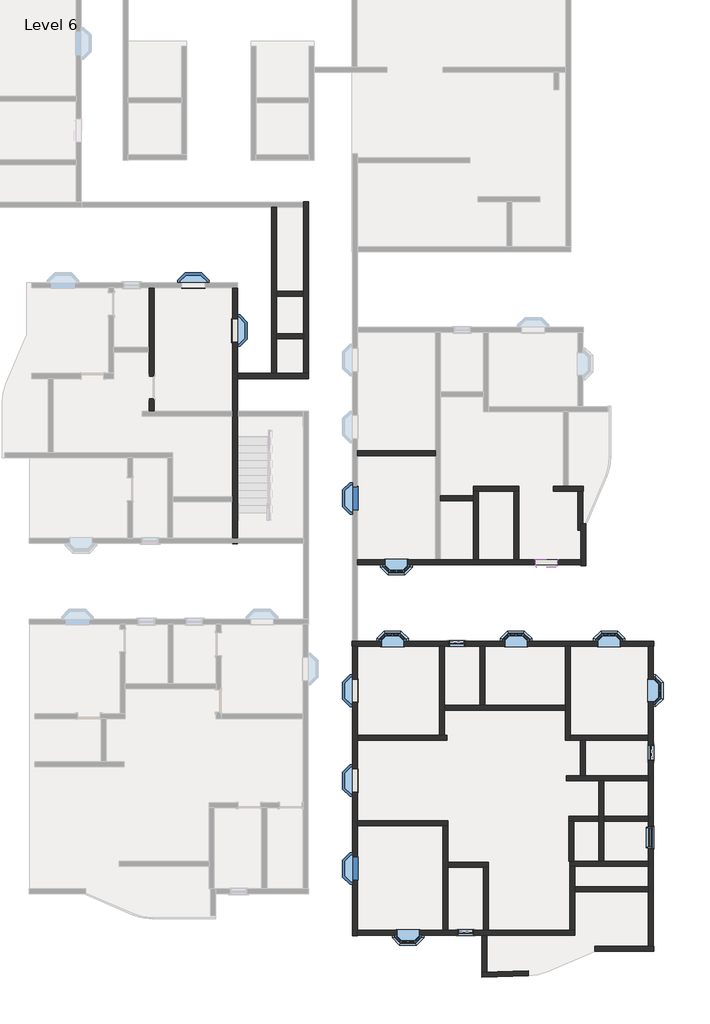
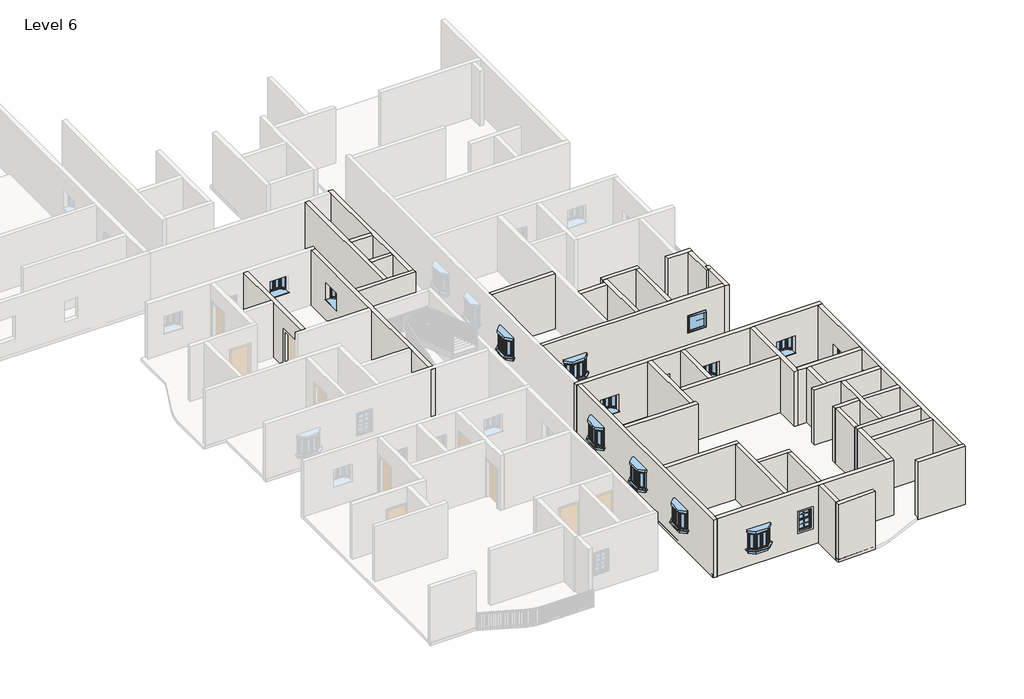
# One storey, part 2 of 14: 41 walls, 17 windows.
# Revit data of these elements (continued)
# Element 41 (IfcWall, "9\" w") (continued)
#   Phase Created = New Construction
#   Base Constraint = Level 6
#   Top Constraint = Level 7
#   Materials on its faces: "Default Wall", "Acoustic Ceiling Tile 24 x 24"
# Element 42 (IfcWindow, "910x910mm")
#   Mark = "314"
#   Phase Created = New Construction
#   Materials on its faces: "Window Frame", "Glass"
# Element 43 (IfcWindow, "910x910mm")
#   Mark = "316"
#   Phase Created = New Construction
#   Materials on its faces: "Window Frame", "Glass"
# Element 44 (IfcWindow, "910x910mm")
#   Mark = "334"
#   Phase Created = New Construction
#   Materials on its faces: "Window Frame", "Glass"
# Element 45 (IfcWindow, "910x910mm")
#   Mark = "325"
#   Phase Created = New Construction
#   Materials on its faces: "Window Frame", "Glass"
# Element 46 (IfcWindow, "910x910mm")
#   Mark = "326"
#   Phase Created = New Construction
#   Materials on its faces: "Window Frame", "Glass"
# Element 47 (IfcWindow, "910x910mm")
#   Mark = "327"
#   Phase Created = New Construction
#   Materials on its faces: "Window Frame", "Glass"
# Element 48 (IfcWindow, "910x910mm")
#   Mark = "328"
#   Phase Created = New Construction
#   Materials on its faces: "Window Frame", "Glass"
# Element 49 (IfcWindow, "910x910mm")
#   Mark = "329"
#   Phase Created = New Construction
#   Materials on its faces: "Window Frame", "Glass"
# Element 50 (IfcWindow, "910x910mm")
#   Mark = "330"
#   Phase Created = New Construction
#   Materials on its faces: "Window Frame", "Glass"
# Element 51 (IfcWindow, "910x910mm")
#   Mark = "331"
#   Phase Created = New Construction
#   Materials on its faces: "Window Frame", "Glass"
# Element 52 (IfcWindow, "910x910mm")
#   Mark = "332"
#   Phase Created = New Construction
#   Materials on its faces: "Window Frame", "Glass"
# Element 53 (IfcWindow, "910x910mm")
#   Mark = "333"
#   Phase Created = New Construction
#   Materials on its faces: "Window Frame", "Glass"
# Element 54 (IfcWindow, "Window-Double-Hung : 26\" x 42\"")
#   Mark = "356"
#   Window Inset = 0' - 0"
#   Interior Wall Closure = 0' - 1 1/2"
#   Frame Extension = 0' - 1 1/4"
#   Exterior Wall Closure = 0' - 0 1/2"
#   Interior Trim Visibility = yes
#   Indicator Visibility = yes
#   Exterior Trim Visibility = yes
#   Phase Created = New Construction
#   Materials on its faces: "Wood - Stained", "Glass", "Clad - White"
# Element 55 (IfcWindow, "Window-Double-Hung : 26\" x 42\"")
#   Mark = "357"
#   Window Inset = 0' - 0"
#   Interior Wall Closure = 0' - 1 1/2"
#   Frame Extension = 0' - 1 1/4"
#   Exterior Wall Closure = 0' - 0 1/2"
#   Interior Trim Visibility = yes
#   Indicator Visibility = yes
#   Exterior Trim Visibility = yes
#   Phase Created = New Construction
#   Materials on its faces: "Wood - Stained", "Glass", "Clad - White"
# Element 56 (IfcWindow, "Window-Double-Hung : 26\" x 42\"")
#   Mark = "358"
#   Window Inset = 0' - 0"
#   Interior Wall Closure = 0' - 1 1/2"
#   Frame Extension = 0' - 1 1/4"
#   Exterior Wall Closure = 0' - 0 1/2"
#   Interior Trim Visibility = yes
#   Indicator Visibility = yes
#   Exterior Trim Visibility = yes
#   Phase Created = New Construction
#   Materials on its faces: "Wood - Stained", "Glass", "Clad - White"
# Element 57 (IfcWindow, "Windows_Sgl_w-Glazing_Bars : 910x910mm")
#   Mark = "346"
#   Phase Created = New Construction
#   Materials on its faces: "Window Frame", "Glass"
# Element 58 (IfcWindow, "Windows_Sgl_w-Glazing_Bars : 910x910mm")
#   Mark = "345"
#   Phase Created = New Construction
#   Materials on its faces: "Window Frame", "Glass"
# Materials
#   "Window Frame": colour RGB 249 249 249, transparency 0
#   "Glass": class "Glass", colour RGB 0 128 192, transparency 0.75, Description = "Soda Lime Glass", Cost = 0
#   "Wood - Stained": class "Wood", colour RGB 224 178 126, transparency 0, Cost = 0
#   "Clad - White": class "Wood", colour RGB 242 242 238, transparency 0, Cost = 0
#   "Default Wall": colour RGB 128 128 128, transparency 0, Cost = 0
#   "Carpet (1)": class "Carpet", colour RGB 124 80 67, transparency 0, Description = "Interior finish", Cost = 0
#   "Door - Frame": colour RGB 118 70 51, transparency 0, Cost = 0
#   "Earth": class "Generic", colour RGB 97 75 62, transparency 0, Description = "Soil", Cost = 0
#   "Acoustic Ceiling Tile 24 x 24": class "Generic", colour RGB 232 232 232, transparency 0, Description = "Acoustic Ceiling Tile 24 x 24", Cost = 0
